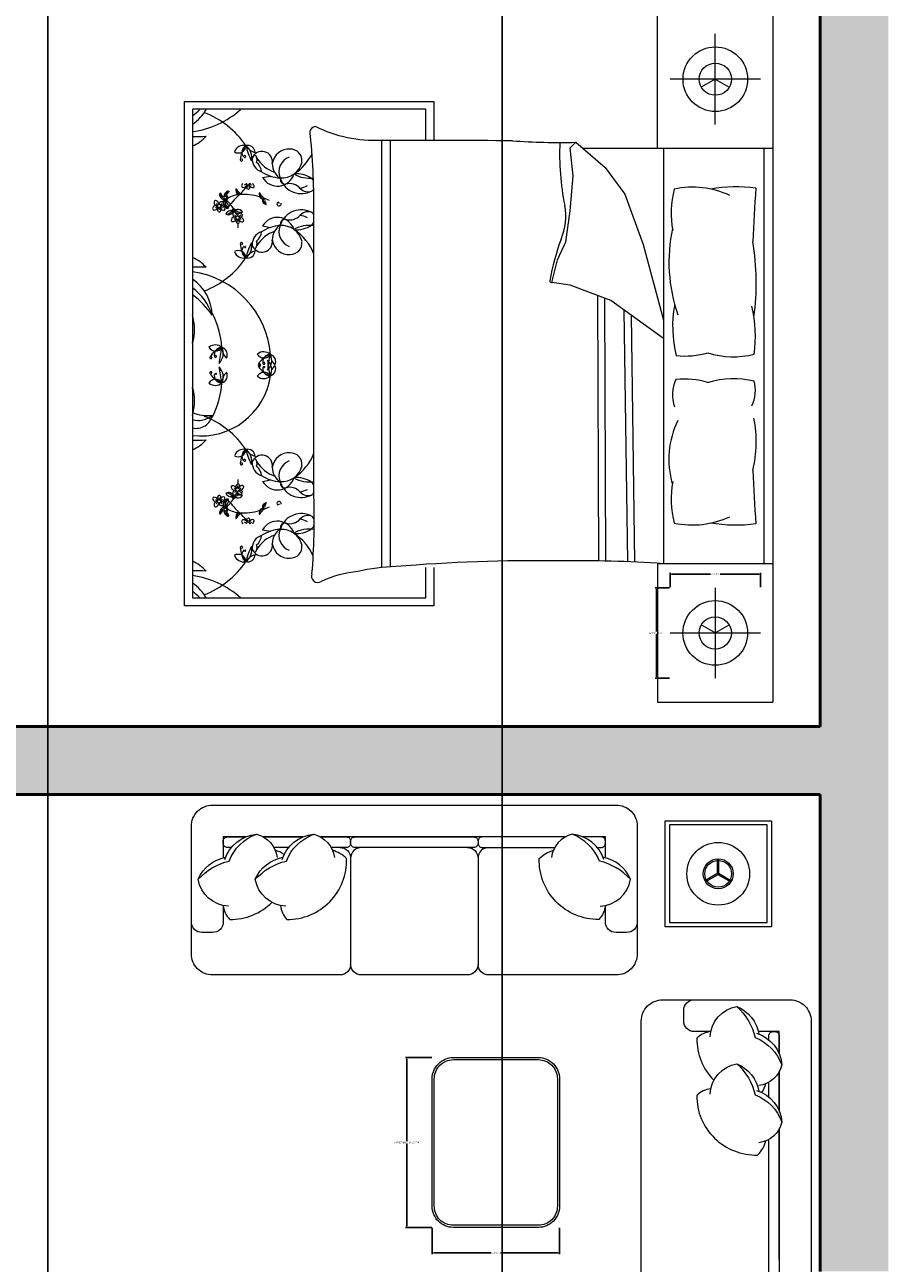
# Model space of a CAD drawing. Units: inches. Extents: x -12 to 604, y -566 to 58.
# Tile 6 of 12: x 166 to 280, y -189 to -25. Entities that reach past the tile are written whole.
import ezdxf

# ---------------------------------------------------------------- set-up
doc = ezdxf.new("R2010")
doc.units = ezdxf.units.IN
doc.header["$MEASUREMENT"] = 0
for name, color, linetype, lineweight in [('A-ANNO-DIMS', 2, 'Continuous', 18), ('A-FURN', 8, 'Continuous', 18), ('A-WALL', 7, 'Continuous', 50), ('A-WALL-PATT', 18, 'Continuous', 13)]:
    doc.layers.add(name, color=color, linetype=linetype, lineweight=lineweight)
doc.styles.get("Standard").update_dxf_attribs({"font": 'arial.ttf'})
doc.dimstyles.get("Standard").update_dxf_attribs({"dimtxt": 0.18, "dimasz": 0.18, "dimexe": 0.18, "dimexo": 0.0625, "dimgap": 0.09, "dimtad": 0, "dimtih": 1, "dimtoh": 1, "dimdec": 0, "dimzin": 0, "dimdsep": 46, "dimlunit": 3, "dimtxsty": 'Standard', "dimcen": 0.09, "dimadec": 0, "dimazin": 0, "dimtfac": 1, "dimtdec": 0, "dimtofl": 0, "dimtmove": 0, "dimatfit": 3, "dimfxl": 1, "dimtolj": 1, "dimtzin": 0, "dimarcsym": 0})

# ---------------------------------------------------------------- blocks, each defined once
blk = doc.blocks.new('DAY BED1')
at = {"color": 0}
blk.add_line((0.3, 0.25), (0.225, 0.2549), dxfattribs=at)
blk.add_lwpolyline([(-0.3, 0, -0.414214), (-0.4, 0.1), (-0.4, 0.1, 0.317837), (-0.4, 0.1, -0.414214), (-0.4, 0.1), (-0.4, 0.1, 1.186185), (-0.4, 0.1, -0.414214), (-0.4, 0.1), (-0.4, 1.5, -0.414214), (-0.3, 1.6), (0.3, 1.6, -0.414214), (0.4, 1.5), (0.4, 0.1, -0.414214), (0.3, 0)], format="xyb", close=True, dxfattribs=at)
for points in [[(-0.0725, 1.45), (-0.15, 1.45, -0.414214), (-0.2, 1.5), (-0.2, 1.55, -0.414214), (-0.15, 1.6)], [(-0.0756, 1.4249, -0.356772), (0.0505, 1.5682, -0.249542), (0.1543, 1.4384, 9.61688)], [(0.0505, 1.5682, -0.14773), (0.1364, 1.422, -0.213343), (0.2624, 1.2931, -0.178662)], [(-0.0725, 1.4501, 0.165541), (-0.1386, 1.4192, 0.200231), (-0.0581, 1.2207, 0.121523)], [(0.1433, 1.4422, -0.306663), (0.2624, 1.2931, -0.30633), (0.1536, 1.1957, 0.872847)], [(0.25, 1.3448), (0.25, 1.45), (0.1517, 1.45, -0.414214)], [(0.2, 1.4118), (0.2, 1.43, -0.414214), (0.22, 1.45), (0.23, 1.45, -0.414214), (0.25, 1.43)], [(0.25, 1.43), (0.25, 1.3448, -0.414214)], [(-0.0756, 1.1556, -0.356772), (0.0505, 1.2988, -0.249542), (0.1543, 1.169, 9.61688)], [(0.0505, 1.2988, -0.14773), (0.1364, 1.1527, -0.213343), (0.2624, 1.0238, -0.178662)], [(0.25, 1.2616), (0.25, 1.0755, -0.414214)], [(-0.0725, 1.1808, 0.165541), (-0.1386, 1.1498, 0.425989), (0.1479, 0.869, 0.121523), (0.1873, 0.9357, -7.115464)], [(0.1433, 1.1729, -0.306663), (0.2624, 1.0238, -0.30633), (0.1536, 0.9263, 0.872847)], [(0.1678, 1.1631, 0.071865), (0.1873, 1.205, -7.115464)], [(0.2, 1.1425), (0.2, 1.2113, -0.414214)], [(0.25, 0.9923), (0.25, 0.2749, -0.414214), (0.23, 0.2549), (0.22, 0.2549, -0.414214), (0.2, 0.2749), (0.2, 0.9419, -0.414214)], [(0.25, 0.3775), (0.25, 0.3, 0.414214), (0.3, 0.25), (0.35, 0.25, 0.414214), (0.4, 0.3)]]:
    blk.add_lwpolyline(points, format="xyb", dxfattribs=at)
for points in [[(0.25, 1.0755), (0.25, 1.2616)], [(0.25, 0.3775), (0.25, 0.9923)]]:
    blk.add_lwpolyline(points, dxfattribs=at)
blk = doc.blocks.new('SIDE-TABLE-WITH-LAMP')
for p, q in [((6.94, 7.06), (7.93, 8.77)), ((7.09, 6.97), (8.08, 8.68)), ((7.01, 7.1), (5.03, 7.1)), ((7.01, 6.92), (5.03, 6.92)), ((6.94, 6.97), (7.93, 5.26)), ((7.09, 7.06), (8.08, 5.34))]:
    blk.add_line(p, q)
at = {"ltscale": 0.03}
blk.add_lwpolyline([(14.03, 14.03), (14.03, 0), (0, 0), (0, 14.03)], close=True, dxfattribs=at)
blk.add_lwpolyline([(13.46, 0.56), (13.46, 13.46), (0.56, 13.46), (0.56, 0.56)], close=True)
for radius in [4.14, 1.98, 1.77]:
    blk.add_circle((7.01, 7.01), radius)
blk = doc.blocks.new('BEDSIDE-LAMP-217')
for p, q in [((5.97, 11.95), (5.97, 0)), ((0, 5.97), (11.95, 5.97))]:
    blk.add_line(p, q)
for points in [[(5.97, 5.97), (4.13, 7.04)], [(5.97, 5.97), (7.82, 7.04)]]:
    blk.add_lwpolyline(points)
for radius in [4.27, 2.13]:
    blk.add_circle((5.97, 5.97), radius)
blk = doc.blocks.new('COFFEE-TABLE')
at = {"ltscale": 0.03}
for points in [[(0, 2.81), (0, 14.03, -0.414214), (2.81, 16.83), (19.64, 16.83, -0.414214), (22.44, 14.03), (22.44, 2.81, -0.414214), (19.64, 0), (2.81, 0, -0.414214)], [(0.28, 2.81), (0.28, 14.03, -0.414214), (2.81, 16.55), (19.64, 16.55, -0.414214), (22.16, 14.03), (22.16, 2.81, -0.414214), (19.64, 0.28), (2.81, 0.28, -0.414214)]]:
    blk.add_lwpolyline(points, format="xyb", close=True, dxfattribs=at)
blk = doc.blocks.new('*D39')
at = {"layer": 'A-ANNO-DIMS', "color": 0, "lineweight": -2, "transparency": 16777216}
for p, q in [((251.44, -99.54), (249.53, -99.54)), ((249.71, -99.72), (249.71, -105.33)), ((249.71, -111.31), (249.71, -105.69)), ((251.44, -111.49), (249.53, -111.49))]:
    blk.add_line(p, q, dxfattribs=at)
at = {"layer": 'A-ANNO-DIMS', "color": 0, "transparency": 16777216}
for points in [[(249.68, -99.72), (249.74, -99.72), (249.71, -99.54)], [(249.68, -111.31), (249.74, -111.31), (249.71, -111.49)]]:
    blk.add_solid(points, dxfattribs=at)
at = {"layer": 'Defpoints', "color": 0, "transparency": 16777216}
for p in [(249.71, -99.54), (251.5, -99.54), (251.5, -111.49)]:
    blk.add_point(p, dxfattribs=at)
at = {"layer": 'A-ANNO-DIMS', "color": 0, "transparency": 16777216, "insert": (249.71, -105.51), "char_height": 0.18, "attachment_point": 5}
blk.add_mtext('\\A1;LAMP B 1\'-0" TYP.', dxfattribs=at)
blk = doc.blocks.new('*D40')
at = {"layer": 'A-ANNO-DIMS', "color": 0, "lineweight": -2, "transparency": 16777216}
for p, q in [((251.5, -99.48), (251.5, -97.57)), ((251.68, -97.75), (256.85, -97.75)), ((263.27, -97.75), (258.11, -97.75)), ((263.45, -99.48), (263.45, -97.57))]:
    blk.add_line(p, q, dxfattribs=at)
at = {"layer": 'A-ANNO-DIMS', "color": 0, "transparency": 16777216}
for points in [[(251.68, -97.72), (251.68, -97.78), (251.5, -97.75)], [(263.27, -97.72), (263.27, -97.78), (263.45, -97.75)]]:
    blk.add_solid(points, dxfattribs=at)
at = {"layer": 'Defpoints', "color": 0, "transparency": 16777216}
for p in [(263.45, -97.75), (251.5, -99.54), (263.45, -99.54)]:
    blk.add_point(p, dxfattribs=at)
at = {"layer": 'A-ANNO-DIMS', "color": 0, "transparency": 16777216, "insert": (257.48, -97.75), "char_height": 0.18, "attachment_point": 5}
blk.add_mtext('\\A1;1\'-0" TYP.', dxfattribs=at)
blk = doc.blocks.new('*D47')
at = {"layer": 'A-ANNO-DIMS', "color": 0, "lineweight": -2, "transparency": 16777216}
for p, q in [((220.01, -161.6), (216.53, -161.6)), ((216.71, -161.78), (216.71, -172.64)), ((216.71, -183.86), (216.71, -173.01)), ((220.01, -184.04), (216.53, -184.04))]:
    blk.add_line(p, q, dxfattribs=at)
at = {"layer": 'A-ANNO-DIMS', "color": 0, "transparency": 16777216}
for points in [[(216.68, -161.78), (216.74, -161.78), (216.71, -161.6)], [(216.68, -183.86), (216.74, -183.86), (216.71, -184.04)]]:
    blk.add_solid(points, dxfattribs=at)
at = {"layer": 'Defpoints', "color": 0, "transparency": 16777216}
for p in [(220.07, -161.6), (216.71, -184.04), (220.07, -184.04)]:
    blk.add_point(p, dxfattribs=at)
at = {"layer": 'A-ANNO-DIMS', "color": 0, "transparency": 16777216, "insert": (216.71, -172.82), "char_height": 0.18, "attachment_point": 5}
blk.add_mtext('\\A1;COFFEE TABLE 1\'-10 1/2" TYP.', dxfattribs=at)
blk = doc.blocks.new('*D48')
at = {"layer": 'A-ANNO-DIMS', "color": 0, "lineweight": -2, "transparency": 16777216}
for p, q in [((220.07, -184.11), (220.07, -187.59)), ((236.91, -184.11), (236.91, -187.59)), ((220.25, -187.41), (227.86, -187.41)), ((236.73, -187.41), (229.12, -187.41))]:
    blk.add_line(p, q, dxfattribs=at)
at = {"layer": 'A-ANNO-DIMS', "color": 0, "transparency": 16777216}
for points in [[(220.25, -187.38), (220.25, -187.44), (220.07, -187.41)], [(236.73, -187.38), (236.73, -187.44), (236.91, -187.41)]]:
    blk.add_solid(points, dxfattribs=at)
at = {"layer": 'Defpoints', "color": 0, "transparency": 16777216}
for p in [(220.07, -184.04), (236.91, -184.04), (236.91, -187.41)]:
    blk.add_point(p, dxfattribs=at)
at = {"layer": 'A-ANNO-DIMS', "color": 0, "transparency": 16777216, "insert": (228.49, -187.41), "char_height": 0.18, "attachment_point": 5}
blk.add_mtext('\\A1;1\'-5" TYP.', dxfattribs=at)
blk = doc.blocks.new('*D57')
at = {"layer": 'A-ANNO-DIMS', "color": 0, "lineweight": -2, "transparency": 16777216}
for p, q in [((169.32, 12.58), (169.32, -565.59)), ((229.32, 12.58), (229.32, -565.59)), ((169.5, -565.41), (198.99, -565.41)), ((229.14, -565.41), (199.65, -565.41))]:
    blk.add_line(p, q, dxfattribs=at)
at = {"layer": 'A-ANNO-DIMS', "color": 0, "transparency": 16777216}
for points in [[(169.5, -565.38), (169.5, -565.44), (169.32, -565.41)], [(229.14, -565.38), (229.14, -565.44), (229.32, -565.41)]]:
    blk.add_solid(points, dxfattribs=at)
at = {"layer": 'Defpoints', "color": 0, "transparency": 16777216}
for p in [(169.32, 12.64), (229.32, 12.64), (229.32, -565.41)]:
    blk.add_point(p, dxfattribs=at)
at = {"layer": 'A-ANNO-DIMS', "color": 0, "transparency": 16777216, "insert": (199.32, -565.41), "char_height": 0.18, "attachment_point": 5}
blk.add_mtext('\\A1;5\'-0"', dxfattribs=at)

msp = doc.modelspace()

# ---------------------------------------------------------------- hatches: boundary and pattern name
at = {"layer": 'A-WALL-PATT'}
h = msp.add_hatch(color=256, dxfattribs=at)
h.dxf.hatch_style = 1
h.paths.add_polyline_path([(169.32, 11.14), (169.32, 17.14), (160.32, 17.14), (160.32, 11.14), (118.32, 11.14), (118.32, 6.64), (118.32, 2.14), (127.32, 2.14), (169.32, 2.14)])
h.paths.add_polyline_path([(127.32, -13.61), (118.32, -13.61), (118.32, -29.36), (34.82, -29.36), (24.32, -29.36), (24.32, -38.36), (39.32, -38.36), (118.32, -38.36), (118.32, -126.86), (127.32, -126.86), (127.32, -117.86)])
h.paths.add_polyline_path([(82.32, -92.36), (39.32, -92.36), (39.32, -56.22), (30.32, -56.22), (24.32, -56.22), (24.32, -65.22), (30.32, -65.22), (30.32, -113.36), (24.32, -113.36), (24.32, -122.36), (39.32, -122.36), (39.32, -101.36), (82.32, -101.36), (82.32, -96.86)], flags=17)
h.paths.add_polyline_path([(280.32, 11.14), (238.32, 11.14), (238.32, 17.14), (229.32, 17.14), (229.32, 12.64), (229.32, 11.14), (229.32, 2.14), (271.32, 2.14), (271.32, -117.86), (163.32, -117.86), (163.32, -126.86), (271.32, -126.86), (271.32, -189.86), (280.32, -189.86), (280.32, -180.86)])
h.paths.add_polyline_path([(415.32, 17.14), (406.32, 17.14), (406.32, 11.14), (358.32, 11.14), (358.32, -21.86), (367.32, -21.86), (367.32, 2.14), (415.32, 2.14)], flags=17)
h.paths.add_polyline_path([(484.55, -45.86), (448.32, -45.86), (448.32, 2.14), (448.32, 17.14), (439.32, 17.14), (439.32, 12.64), (439.32, 2.14), (439.32, -45.86), (367.32, -45.86), (358.32, -45.86), (358.32, -54.86), (430.32, -54.86), (430.32, -69.59), (430.32, -180.86), (318.82, -180.86), (318.82, -189.86), (318.82, -331.86), (327.82, -331.86), (327.82, -189.86), (439.32, -189.86), (439.32, -180.86), (439.32, -54.86), (483.5, -54.86), (484.55, -54.86)])
h.paths.add_polyline_path([(529.32, 11.14), (481.32, 11.14), (481.32, 17.14), (472.32, 17.14), (472.32, 12.64), (472.32, 2.14), (520.32, 2.14), (520.32, -21.86), (529.32, -21.86)])
h.paths.add_polyline_path([(598.32, -45.86), (582.42, -45.86), (582.42, -50.36), (582.42, -54.86), (589.32, -54.86), (589.32, -99.86), (598.32, -99.86), (604.32, -99.86), (604.32, -90.86), (598.32, -90.86)])
h.paths.add_polyline_path([(598.32, -168.86), (604.32, -168.86), (604.32, -159.86), (589.32, -159.86), (589.32, -180.86), (477.32, -180.86), (477.32, -189.86), (477.32, -259.86), (486.32, -259.86), (486.32, -189.86), (589.32, -189.86), (589.32, -204.86), (598.32, -204.86), (604.32, -204.86), (604.32, -195.86), (598.32, -195.86)])
h.paths.add_polyline_path([(598.32, -244.86), (604.32, -244.86), (604.32, -235.86), (598.32, -235.86), (589.32, -235.86), (589.32, -250.86), (522.32, -250.86), (522.32, -259.86), (589.32, -259.86), (589.32, -274.86), (598.32, -274.86), (604.32, -274.86), (604.32, -265.86), (598.32, -265.86)])
h.paths.add_polyline_path([(598.32, -333.28), (604.32, -333.28), (604.32, -324.28), (598.32, -324.28), (598.32, -321.87), (598.32, -318.28), (604.32, -318.28), (604.32, -309.28), (598.32, -309.28), (589.32, -309.28), (589.32, -341.95), (589.38, -341.95), (589.38, -363.16), (589.32, -381.86), (565.32, -381.86), (565.32, -390.86), (589.32, -390.86), (589.32, -450.86), (598.32, -450.86), (604.32, -450.86), (604.32, -441.86), (598.32, -441.86), (598.32, -390.86), (604.32, -390.86), (604.32, -381.86), (598.32, -381.86)])
h.paths.add_polyline_path([(541.32, -345.86), (424.32, -345.86), (424.32, -354.86), (532.32, -354.86), (532.32, -474.86), (463.39, -474.86), (463.39, -483.86), (553.32, -483.86), (553.32, -474.86), (541.32, -474.86), (541.32, -390.86), (541.32, -381.86)])
h.paths.add_polyline_path([(604.32, -474.86), (589.32, -474.86), (553.32, -474.86), (553.32, -483.86), (598.32, -483.86), (604.32, -483.86)])
h.paths.add_polyline_path([(388.32, -483.86), (388.32, -474.86), (388.32, -460.13), (388.32, -333.86), (388.32, -322.86), (379.32, -322.86), (379.32, -331.86), (379.32, -333.86), (379.32, -474.86), (379.32, -520.86), (344.32, -520.86), (344.32, -529.86), (379.32, -529.86), (388.32, -529.86)])
h.paths.add_polyline_path([(284.32, -520.86), (249.32, -520.86), (249.32, -474.86), (249.32, -368.36), (240.32, -368.36), (240.32, -474.86), (238.52, -474.86), (238.52, -483.86), (240.32, -483.86), (240.32, -529.86), (249.32, -529.86), (284.32, -529.86)])
h.paths.add_polyline_path([(178.82, -474.86), (158.91, -474.86), (158.91, -483.86), (162.32, -483.86), (178.82, -483.86)])
h.paths.add_polyline_path([(84.32, -474.86), (84.32, -366.86), (75.32, -366.86), (75.32, -474.86), (39.32, -474.86), (39.32, -453.86), (24.32, -453.86), (24.32, -462.86), (30.32, -462.86), (30.32, -483.86), (84.32, -483.86)])
h.paths.add_polyline_path([(39.32, -342.86), (75.32, -342.86), (84.32, -342.86), (179.67, -342.86), (179.67, -333.86), (39.32, -333.86), (39.32, -318.86), (24.32, -318.86), (24.32, -327.86), (30.32, -327.86), (30.32, -432.86), (24.32, -432.86), (24.32, -441.86), (30.32, -441.86), (39.32, -441.86)])
h.paths.add_polyline_path([(249.32, -252.86), (115.32, -252.86), (115.32, -225.86), (106.32, -225.86), (106.32, -252.86), (39.32, -252.86), (39.32, -237.86), (24.32, -237.86), (24.32, -246.86), (30.32, -246.86), (30.32, -267.86), (24.32, -267.86), (24.32, -276.86), (39.32, -276.86), (39.32, -261.86), (240.32, -261.86), (240.32, -331.86), (249.32, -331.86), (266.82, -331.86), (266.82, -322.86), (249.32, -322.86)])
h.paths.add_polyline_path([(127.32, -180.86), (39.32, -180.86), (24.32, -180.86), (24.32, -189.86), (39.32, -189.86), (127.32, -189.86)])
h.paths.add_polyline_path([(39.32, -159.86), (24.32, -159.86), (24.32, -168.86), (30.32, -168.86), (30.32, -180.86), (39.32, -180.86)])
h.paths.add_polyline_path([(470.51, -17.27), (512.48, -17.27), (512.48, 5.12), (470.51, 5.12)], flags=9)
h.paths.add_polyline_path([(484.21, -244.26), (526.45, -244.26), (526.45, -221.87), (484.21, -221.87)], flags=24)
h.paths.add_polyline_path([(36.91, -442.88), (83.54, -442.88), (83.54, -420.5), (36.91, -420.5)], flags=25)

# ---------------------------------------------------------------- linework, layer by layer
at = {"layer": 'A-FURN'}
for p, q in [((265.09, -23.23), (265.09, -114.65)), ((187.34, -35.3), (220.28, -35.3)), ((187.34, -101.95), (187.34, -35.3)), ((220.28, -35.3), (220.28, -40.47)), ((188.4, -36.35), (188.4, -100.89)), ((219.22, -36.35), (188.4, -36.35)), ((219.22, -40.46), (219.22, -36.35)), ((213.43, -96.87), (213.43, -40.46)), ((214.57, -96.78), (214.57, -40.46)), ((238.31, -41.44), (239.05, -40.69)), ((239.05, -40.69), (242.93, -44.03)), ((238.68, -45.14), (238.31, -41.44)), ((265.09, -41.51), (240, -41.51)), ((250.65, -41.51), (250.65, -96.37)), ((263.92, -96.37), (263.92, -41.51)), ((242.93, -44.03), (245.52, -47.55)), ((197.67, -45.36), (198.7, -45.16)), ((238.31, -49.77), (238.68, -45.14)), ((245.52, -47.55), (247.93, -54.21)), ((204.45, -87.5), (204.45, -50.38)), ((237.75, -53.84), (238.31, -49.77)), ((197.67, -51.75), (198.7, -51.96)), ((236.64, -56.25), (237.75, -53.84)), ((247.93, -54.21), (250.65, -64.18)), ((235.9, -59.21), (236.64, -56.25)), ((238.31, -59.58), (235.9, -59.21)), ((243.67, -61.62), (238.31, -59.58)), ((242.09, -96.05), (241.95, -60.97)), ((243.03, -96.04), (242.89, -61.32)), ((250.65, -66.63), (243.67, -61.62)), ((245.91, -96.09), (245.44, -62.89)), ((246.85, -96.12), (246.39, -63.57)), ((197.67, -85.49), (198.7, -85.29)), ((197.67, -91.88), (198.7, -92.08)), ((219.22, -100.89), (219.22, -96.86)), ((220.28, -96.88), (220.28, -101.95)), ((188.4, -100.89), (219.22, -100.89)), ((220.28, -101.95), (187.34, -101.95))]:
    msp.add_line(p, q, dxfattribs=at)
for points in [[(249.86, -41.51), (249.86, -23.23), (265.09, -23.23)], [(265.09, -96.37), (249.86, -96.37), (249.86, -114.65), (265.09, -114.65)], [(202.97, -132.46), (197.75, -132.46)], [(237.67, -132.46), (205.31, -132.46)], [(242.96, -135.21), (242.96, -132.46), (240.01, -132.46)]]:
    msp.add_lwpolyline(points, dxfattribs=at)
for points in [[(230.67, -40.5, 0.001242), (213.33, -40.46, -0.127202), (204.68, -38.63)], [(262.82, -46.76, 0.074897), (256.84, -46.88, -0.472817)], [(256.51, -68.51, 0.14099), (262.6, -68.7, 0.235245)], [(256.51, -72.42, -0.14099), (262.6, -72.23, -0.235245)], [(262.82, -91.12, -0.074897), (256.84, -91.01, 0.472817)], [(215.29, -96.76, 0.056112), (210.26, -97.42, 0.095341), (205.42, -98.71)], [(189.15, -138.05, -0.14773), (193.25, -135.64, -0.213343), (196.87, -132.11, -0.178662)], [(195.42, -132.46), (192.47, -132.46), (192.47, -135.21, -0.414214)], [(193.54, -133.86), (193.03, -133.86, -0.414214), (192.47, -133.3), (192.47, -133.02, -0.414214), (193.03, -132.46)], [(192.68, -135.45, -0.306663), (196.87, -132.11, -0.30633), (199.6, -135.16, 0.872847)], [(193.03, -132.46), (195.42, -132.46, -0.414214)], [(196.71, -138.05, -0.14773), (200.81, -135.64, -0.213343), (204.42, -132.11, -0.178662)], [(197.75, -132.46), (202.97, -132.46, -0.414214)], [(200.24, -135.45, -0.306663), (204.42, -132.11, -0.30633), (207.16, -135.16, 0.872847)], [(205.31, -132.46), (208.74, -132.46, -0.414214), (209.3, -133.02), (209.3, -133.3, -0.414214), (208.74, -133.86), (206.72, -133.86, -0.414214)], [(237.67, -132.46), (226.69, -132.46, 0.414214), (226.13, -133.02), (226.13, -133.3, 0.414214), (226.69, -133.86), (236.26, -133.86, 0.414214)], [(242.74, -135.45, 0.306663), (238.56, -132.11, 0.30633), (235.82, -135.16, -0.872847)], [(246.27, -138.05, 0.14773), (242.17, -135.64, 0.213343), (238.56, -132.11, 0.178662)], [(242.4, -132.46), (240.01, -132.46, 0.414214)], [(241.89, -133.86), (242.4, -133.86, 0.414214), (242.96, -133.3), (242.96, -133.02, 0.414214), (242.4, -132.46)], [(201.09, -133.86), (199.16, -133.86, -0.414214)], [(207.89, -133.86, -0.414214), (209.3, -135.26), (209.3, -149.29, -0.414214)], [(210.7, -133.86, 0.414214), (209.3, -135.26)], [(224.72, -133.86, -0.414214), (226.13, -135.26)], [(227.53, -133.86, 0.414214), (226.13, -135.26), (226.13, -149.29, 0.414214)], [(193.17, -141.59, -0.356772), (189.15, -138.05, -0.249542), (192.79, -135.14, 9.61688)], [(200.73, -141.59, -0.356772), (196.71, -138.05, -0.249542), (200.35, -135.14, 9.61688)], [(200.51, -134.76, 0.071865), (199.34, -134.22, -7.115464)], [(200.02, -141.5, 0.165541), (200.89, -143.36, 0.425989), (208.76, -135.32, 0.121523), (206.89, -134.22, -7.115464)], [(242.96, -141.5, -0.165541), (242.09, -143.36, -0.425989), (234.22, -135.32, -0.121523), (236.09, -134.22, 7.115464)], [(242.25, -141.59, 0.356772), (246.27, -138.05, 0.249542), (242.63, -135.14, -9.61688)], [(192.47, -141.51), (192.47, -143.68, -0.414214), (191.06, -145.08), (189.66, -145.08, -0.414214), (188.26, -143.68)], [(192.46, -141.5, 0.165541), (193.33, -143.36, 0.200231), (198.9, -141.1, 0.121523)], [(247.17, -143.68, -0.414214), (245.76, -145.08), (244.36, -145.08, -0.414214), (242.96, -143.68), (242.96, -141.51)]]:
    msp.add_lwpolyline(points, format="xyb", dxfattribs=at)
at = {"layer": 'A-FURN', "ltscale": 0.03}
msp.add_lwpolyline([(247.17, -147.89, -0.414214), (244.36, -150.69), (227.53, -150.69, -0.414214), (226.13, -149.29, -0.414214), (224.72, -150.69), (210.7, -150.69, -0.414214), (209.3, -149.29, -0.414214), (207.89, -150.69), (191.06, -150.69, -0.414214), (188.26, -147.89), (188.26, -131.06, -0.414214), (191.06, -128.25), (244.36, -128.25, -0.414214), (247.17, -131.06)], format="xyb", close=True, dxfattribs=at)
at = {"layer": 'A-FURN'}
msp.add_lwpolyline([(209.86, -132.46), (225.57, -132.46, -0.414214), (226.13, -133.02), (226.13, -133.3, -0.414214), (225.57, -133.86), (209.86, -133.86, -0.414214), (209.3, -133.3), (209.3, -133.02, -0.414214)], format="xyb", close=True, dxfattribs=at)
for centre in [(191.9, -49.12), (194.36, -50.65), (194.36, -86.6), (191.9, -88.12)]:
    msp.add_circle(centre, 0.233, dxfattribs=at)
for centre, radius, start, end in [((184.11, -31.36), 7.25, 306.3036, 316.4814), ((185.19, -33.46), 5.82, 303.4617, 330.1116), ((186.79, -27.47), 11.94, 277.745, 311.8856), ((185.61, -47.89), 11.94, 34.3865, 68.5908), ((204.74, -39.47), 0.844, 93.98, 207.3412), ((186.54, -36.71), 4.85, 292.5547, 318.9546), ((189.15, -23.42), 16.52, 267.4081, 273.6519), ((109.28, -49.29), 95.18, 359.3433, 5.6887), ((236.77, 43.13), 83.86, 265.8294, 271.553), ((271.42, -42.26), 34.51, 177.4519, 191.3392), ((195.18, -42.44), 1.32, 77.7115, 159.0387), ((194.47, -41.12), 0.997, 238.4633, 358.2869), ((197.74, -43.14), 3.02, 138.8402, 177.9352), ((195.92, -42.01), 0.977, 117.6827, 223.7762), ((195.31, -42.6), 0.129, 223.7762, 159.7183), ((195.7, -42.11), 0.99, 2.9516, 103.728), ((203.62, -39.34), 8.35, 192.5173, 207.1824), ((194.36, -42.68), 1.89, 345.4653, 54.2343), ((197.21, -40.09), 2.04, 211.3827, 255.2969), ((197.6, -43.27), 1.37, 350.264, 160.8688), ((196.11, -42.99), 0.841, 333.9755, 53.2681), ((201.12, -43.78), 2.18, 84.9449, 172.8857), ((201.34, -43.14), 1.54, 354.4856, 91.0538), ((198.02, -39.11), 6.92, 303.6671, 333.2997), ((194.87, -43.03), 0.148, 177.9352, 11.4834), ((194.94, -43.02), 0.072, 11.4834, 127.9409), ((198.01, -42.94), 1.71, 175.969, 254.3045), ((195.73, -44.79), 1.82, 6.1662, 51.5825), ((200.62, -40.55), 4.32, 211.2614, 251.7045), ((201.6, -43.4), 2.66, 182.3591, 234.0401), ((201.95, -44.63), 2.12, 111.5819, 201.4221), ((200.2, -42.67), 2.75, 265.2933, 346.921), ((200.27, -40.51), 4.91, 236.2883, 266.5076), ((199.64, -44.23), 2.27, 209.9085, 343.1337), ((200.6, -45.67), 0.567, 167.3041, 285.1471), ((202.13, -48.39), 3.53, 122.7011, 126.3445), ((202.79, -44.58), 2.91, 199.2822, 299.1751), ((203.78, -41.65), 3.79, 238.8218, 279.1554), ((202.13, -48.39), 3.53, 55.785, 94.7304), ((203.44, -46.34), 1.1, 30.0293, 52.325), ((192.24, -47.62), 0.26, 124.3538, 214.3923), ((192.8, -47.44), 0.704, 176.9701, 248.2913), ((197.82, -43.73), 6.8, 212.6784, 216.3746), ((193.2, -47.8), 0.606, 122.8155, 187.3992), ((193.47, -47.87), 0.704, 109.4799, 177.6828), ((193.09, -47.43), 0.26, 56.8636, 146.9021), ((198.82, -51.09), 6.8, 145.1882, 148.8844), ((196.72, -46.91), 2.58, 178.3264, 187.1302), ((193.94, -47.27), 0.48, 11.3256, 64.4621), ((195.56, -46.58), 1.45, 190.2588, 210.656), ((194.6, -47.17), 0.439, 188.3432, 274.2869), ((194.98, -46.92), 0.766, 210.656, 242.6341), ((195.56, -46.26), 1.47, 218.2101, 226.3071), ((194.47, -47.5), 0.186, 325.7657, 67.4417), ((188.69, -41.27), 8.68, 313.1541, 322.0459), ((195.07, -46.49), 0.179, 142.4737, 265.053), ((195.31, -46.45), 0.384, 127.7621, 169.0403), ((195.11, -46.12), 0.541, 265.053, 338.3618), ((195.82, -46.86), 0.707, 113.4276, 137.6104), ((195.74, -46.13), 0.233, 183.2768, 356.7232), ((195.91, -46.55), 0.381, 139.7889, 227.6792), ((195.79, -46.69), 0.201, 227.6792, 350.3487), ((195.01, -46.55), 0.762, 353.0852, 15.7171), ((195.51, -46.64), 0.481, 350.3487, 43.6538), ((196.41, -46.14), 0.56, 198.7263, 262.5032), ((195.96, -46.4), 0.222, 1.1081, 91.8675), ((196.38, -46.52), 0.18, 255.2356, 54.9248), ((196.1, -46.45), 0.388, 11.5637, 52.6358), ((199.8, -47.45), 2.58, 178.3264, 187.1302), ((197.01, -47.81), 0.48, 11.3256, 64.4621), ((198.64, -47.12), 1.45, 190.2588, 210.656), ((201.23, -48.03), 1.87, 41.5653, 105.1471), ((202.27, -44.14), 2.63, 277.436, 299.9149), ((203.66, -45.88), 1.37, 221.5653, 293.8354), ((203.44, -46.34), 1.1, 314.4517, 333.558), ((263.89, -50.03), 12.25, 165.1039, 191.0369), ((254.45, -58.41), 11.78, 65.1316, 101.7583), ((1132.9, -97.16), 871.54, 176.68521, 177.14978), ((191.47, -49.44), 0.384, 61.2196, 169.0403), ((191.73, -48.65), 0.46, 157.4086, 261.4386), ((191.47, -48.63), 0.231, 58.0499, 135.6268), ((191.71, -48.78), 0.154, 172.906, 277.132), ((191.2, -49.06), 0.734, 14.7558, 58.0499), ((192.23, -48.87), 0.318, 36.1046, 181.4281), ((192.62, -47.66), 0.606, 190.3057, 287.1958), ((192.04, -48.62), 0.32, 270.0645, 331.1507), ((192.32, -48.69), 0.366, 221.8413, 265.7877), ((192.31, -48.83), 0.228, 263.7526, 41.7054), ((192.26, -49.45), 0.388, 11.5637, 86.365), ((192.56, -47.61), 0.269, 216.3746, 291.7548), ((194.94, -51.39), 3.8, 124.0033, 132.4917), ((191.04, -51.87), 4.06, 63.7819, 68.2913), ((193.2, -48.74), 0.645, 128.3208, 208.8162), ((193.32, -48.7), 0.771, 207.7043, 254.3516), ((192.74, -48.05), 0.203, 289.3605, 111.7548), ((192.89, -48.05), 0.203, 221.8703, 44.2646), ((193.81, -48.64), 1.06, 157.2305, 229.0635), ((193.45, -48.29), 0.625, 174.4544, 220.6188), ((189.9, -51.78), 4.55, 30.544, 49.818), ((193.23, -47.72), 0.269, 148.8844, 224.2646), ((192.41, -49.18), 0.751, 340.0041, 40.6188), ((194.94, -51.39), 3.8, 94.756, 119.2041), ((203.03, -56.85), 12.49, 132.2412, 142.1744), ((195.13, -55.16), 7.57, 73.5842, 93.8277), ((197.67, -47.71), 0.439, 188.3432, 274.2869), ((198.06, -47.47), 0.766, 210.656, 242.6341), ((198.64, -46.81), 1.47, 218.2101, 226.3071), ((197.55, -48.04), 0.186, 325.7657, 67.4417), ((198.07, -48.38), 0.439, 147.5332, 233.4768), ((198.47, -48.16), 0.766, 179.1859, 211.164), ((197.72, -48.33), 0.186, 354.3784, 96.0543), ((195.13, -55.16), 7.57, 63.0032, 69.8941), ((199.3, -46.63), 2.58, 234.6898, 243.4936), ((199.05, -47.81), 1.45, 211.164, 231.5612), ((199.33, -47.96), 1.47, 195.5129, 203.6099), ((197.67, -48.92), 0.48, 357.3579, 50.4944), ((199.74, -48.82), 0.176, 12.7051, 190.4384), ((199.84, -48.8), 0.287, 190.4384, 10.4136), ((230.29, -50.51), 7.44, 336.2616, 11.3392), ((191.24, -49.48), 0.179, 142.4737, 265.053), ((191.27, -49.12), 0.541, 265.053, 338.3618), ((191.98, -49.86), 0.707, 113.4276, 137.6104), ((192.07, -49.54), 0.381, 139.7889, 227.6792), ((191.95, -49.68), 0.201, 227.6792, 350.3487), ((191.18, -49.54), 0.762, 353.0852, 15.7171), ((191.68, -49.63), 0.481, 350.3487, 43.6538), ((192.57, -49.13), 0.56, 198.7263, 262.5032), ((192.12, -49.39), 0.222, 1.1081, 91.8675), ((192.54, -49.51), 0.18, 255.2356, 54.9248), ((192.82, -49.14), 1.06, 270.278, 342.111), ((193.53, -50.47), 0.751, 98.7227, 159.3375), ((193.15, -49.5), 0.771, 244.9899, 291.6373), ((193.32, -49.11), 0.625, 278.7227, 324.8872), ((193.21, -49.61), 0.645, 290.5253, 358.5375), ((193.93, -50.96), 0.384, 61.2196, 169.0403), ((194.18, -50.17), 0.46, 157.4086, 261.4386), ((193.92, -50.16), 0.231, 58.0499, 135.6268), ((194.47, -49.43), 0.645, 182.8499, 266.1226), ((194.22, -48.97), 0.625, 231.7607, 277.9252), ((194.7, -48.86), 1.06, 214.5369, 286.3699), ((194.16, -50.3), 0.154, 172.906, 277.132), ((193.65, -50.58), 0.734, 14.7558, 58.0499), ((189.9, -51.78), 4.55, 23.0501, 23.8477), ((194.41, -50.34), 0.751, 37.3105, 97.9252), ((194.68, -50.39), 0.318, 36.1046, 181.4281), ((194.49, -49.31), 0.771, 265.0106, 311.658), ((194.5, -50.14), 0.32, 270.0645, 331.1507), ((194.77, -50.22), 0.366, 221.8413, 265.7877), ((194.58, -50.92), 0.222, 1.1081, 91.8675), ((194.77, -50.35), 0.228, 263.7526, 41.7054), ((194.72, -50.97), 0.388, 11.5637, 86.365), ((199.64, -52.89), 2.27, 16.8663, 150.0915), ((202.79, -52.53), 2.91, 60.8249, 160.7178), ((201.23, -49.09), 1.87, 254.8529, 318.4347), ((202.27, -52.97), 2.63, 60.0851, 82.564), ((203.66, -51.24), 1.37, 66.1646, 138.4347), ((203.44, -50.78), 1.1, 23.229, 45.5483), ((193.69, -51), 0.179, 142.4737, 265.053), ((193.72, -50.64), 0.541, 265.053, 338.3618), ((194.44, -51.38), 0.707, 113.4276, 137.6104), ((194.53, -51.07), 0.381, 139.7889, 227.6792), ((194.41, -51.2), 0.201, 227.6792, 350.3487), ((193.63, -51.06), 0.762, 353.0852, 15.7171), ((189.9, -51.78), 4.55, 357.1071, 4.7585), ((194.13, -51.15), 0.481, 350.3487, 43.6538), ((195.02, -50.66), 0.56, 198.7263, 262.5032), ((195, -51.04), 0.18, 255.2356, 54.9248), ((200.27, -56.61), 4.91, 93.4924, 123.7117), ((201.6, -53.72), 2.66, 125.9599, 177.6409), ((201.95, -52.48), 2.12, 158.5779, 248.4181), ((200.2, -54.45), 2.75, 13.079, 94.7067), ((200.6, -51.45), 0.567, 74.8529, 192.6959), ((202.13, -48.73), 3.53, 233.6555, 237.2989), ((203.78, -55.47), 3.79, 79.7133, 121.1782), ((202.13, -48.73), 3.53, 265.2696, 304.215), ((198.02, -58.01), 6.92, 21.4941, 56.3329), ((203.44, -50.78), 1.1, 307.675, 336.7144), ((272.6, -56.48), 21.25, 168.0397, 199.2615), ((194.87, -54.09), 0.148, 348.5166, 182.0648), ((194.36, -54.44), 1.89, 305.7657, 14.5347), ((203.62, -57.78), 8.35, 152.8176, 167.4827), ((198.01, -54.17), 1.71, 105.6955, 184.031), ((197.6, -53.85), 1.37, 199.1312, 9.736), ((196.11, -54.13), 0.841, 306.7319, 26.0245), ((195.73, -52.33), 1.82, 308.4175, 353.8338), ((200.62, -56.57), 4.32, 108.2955, 148.7386), ((201.12, -53.34), 2.18, 187.1143, 275.0551), ((201.34, -53.98), 1.54, 268.9462, 5.5144), ((270.45, -65.56), 35.46, 160.1194, 169.3383), ((229.73, -59.29), 33.16, 352.2196, 9.497), ((194.47, -56), 0.997, 1.7131, 121.5367), ((195.18, -54.68), 1.32, 200.9613, 282.2885), ((197.74, -53.98), 3.02, 182.0648, 221.1598), ((194.94, -54.1), 0.072, 232.0591, 348.5166), ((195.92, -55.1), 0.977, 136.2238, 242.3173), ((195.36, -54.53), 0.0778, 200.2667, 136.2271), ((195.7, -55.01), 0.99, 256.272, 357.0484), ((197.21, -57.03), 2.04, 104.7031, 148.6173), ((186.54, -60.4), 4.85, 41.0454, 67.4453), ((189.15, -73.7), 16.52, 86.3481, 92.5919), ((185.61, -49.23), 11.94, 291.4092, 325.6135), ((186.79, -69.65), 11.94, 4.4623, 82.255), ((185.19, -63.66), 5.82, 1.272, 56.5383), ((184.11, -65.76), 7.25, 17.8504, 53.6964), ((235.83, -59), 0.221, 178.8623, 289.7536), ((182.07, -69.57), 10.78, 34.0123, 54.053), ((182.12, -65.4), 6.56, 343.5431, 17.0202), ((180.4, -68.74), 11.94, 4.4623, 27.4146), ((267.96, -65.08), 16.12, 169.8617, 193.6238), ((246.49, -66.29), 16.29, 351.5249, 13.96), ((178.74, -68), 9.71, 4.3787, 5.6357), ((172.09, -73.11), 17.35, 19.7217, 19.9028), ((191.41, -68.79), 1.32, 47.7873, 129.1145), ((191.45, -67.29), 0.997, 208.5391, 328.3627), ((193.28, -70.67), 3.02, 108.9159, 148.011), ((192.26, -68.78), 0.977, 87.7585, 193.852), ((200.27, -70.31), 8.35, 162.593, 177.2582), ((190.58, -68.59), 1.89, 315.5411, 24.3101), ((194.34, -67.76), 2.04, 181.4585, 225.3727), ((192.02, -68.76), 0.99, 333.0274, 73.8037), ((197.81, -69.7), 1.32, 47.7873, 129.1145), ((197.85, -68.2), 0.997, 208.5391, 328.3627), ((253.45, -57.74), 11.2, 264.0129, 285.8293), ((190.84, -69.14), 0.148, 148.011, 341.5592), ((190.92, -69.17), 0.072, 341.5592, 98.0167), ((191.44, -68.99), 0.129, 193.852, 129.9245), ((197.24, -70.06), 0.148, 148.011, 341.5592), ((197.24, -70.23), 0.148, 18.4408, 211.989), ((199.67, -71.58), 3.02, 108.9159, 148.011), ((199.67, -68.71), 3.02, 211.989, 251.0841), ((197.31, -70.08), 0.072, 341.5592, 98.0167), ((197.31, -70.21), 0.072, 261.9833, 18.4408), ((198.66, -69.7), 0.977, 87.7585, 193.852), ((197.83, -69.9), 0.129, 193.852, 129.9245), ((197.88, -70.38), 0.0778, 230.1909, 166.0209), ((196.98, -69.5), 1.89, 315.5411, 24.3101), ((206.67, -71.22), 8.35, 162.593, 177.2582), ((196.98, -70.79), 1.89, 335.6899, 44.4589), ((206.67, -69.07), 8.35, 182.7418, 197.407), ((198.42, -69.67), 0.99, 333.0274, 73.8037), ((200.73, -68.67), 2.04, 181.4585, 225.3727), ((198.42, -70.62), 0.99, 286.1963, 26.9726), ((200.73, -71.62), 2.04, 134.6273, 178.5415), ((189.55, -70.25), 9.24, 262.8636, 351.8197), ((190.84, -71.15), 0.148, 18.4408, 211.989), ((193.28, -69.63), 3.02, 211.989, 251.0841), ((190.92, -71.12), 0.072, 261.9833, 18.4408), ((192.26, -71.51), 0.977, 166.148, 272.2415), ((191.49, -71.29), 0.0778, 230.1909, 166.0209), ((200.27, -69.98), 8.35, 182.7418, 197.407), ((190.58, -71.71), 1.89, 335.6899, 44.4589), ((194.34, -72.53), 2.04, 134.6273, 178.5415), ((192.02, -71.53), 0.99, 286.1963, 26.9726), ((197.85, -72.09), 0.997, 31.6373, 151.4609), ((197.81, -70.59), 1.32, 230.8855, 312.2127), ((198.66, -70.59), 0.977, 166.148, 272.2415), ((182.12, -74.89), 6.56, 342.9798, 16.4569), ((178.74, -72.29), 9.71, 354.3643, 355.6213), ((172.09, -67.18), 17.35, 340.0972, 340.2783), ((191.45, -73.01), 0.997, 31.6373, 151.4609), ((191.41, -71.5), 1.32, 230.8855, 312.2127), ((180.4, -71.55), 11.94, 332.5854, 355.5377), ((256.68, -74.1), 4.85, 155.0183, 198.5407), ((253.45, -83.19), 11.2, 74.1707, 95.9871), ((258.26, -73.49), 4.52, 333.3437, 16.1026), ((190.39, -71.45), 5.35, 248.117, 276.6195), ((188.91, -76.35), 2.14, 256.3898, 349.0739), ((189.2, -74.74), 2.71, 252.8609, 311.9049), ((185.61, -88.02), 11.94, 34.3865, 68.5908), ((262.98, -82.57), 11.64, 153.8761, 196.1746), ((246.82, -80.27), 16.07, 346.3427, 11.1841), ((189.15, -63.54), 16.52, 267.4081, 273.6519), ((186.54, -76.84), 4.85, 292.5547, 318.9546), ((195.18, -82.57), 1.32, 77.7115, 159.0387), ((194.47, -81.25), 0.997, 238.4633, 358.2869), ((197.74, -83.26), 3.02, 138.8402, 177.9352), ((195.92, -82.14), 0.977, 117.6827, 223.7762), ((195.7, -82.24), 0.99, 2.9516, 103.728), ((197.21, -80.21), 2.04, 211.3827, 255.2969), ((194.36, -82.81), 1.89, 345.4653, 54.2343), ((203.62, -79.47), 8.35, 192.5173, 207.1824), ((201.12, -83.9), 2.18, 84.9449, 172.8857), ((201.34, -83.27), 1.54, 354.4856, 91.0538), ((198.02, -79.24), 6.92, 303.6671, 338.5059), ((194.87, -83.16), 0.148, 177.9352, 11.4834), ((194.94, -83.14), 0.072, 11.4834, 127.9409), ((195.31, -82.73), 0.129, 223.7762, 159.7183), ((197.6, -83.4), 1.37, 350.264, 160.8688), ((198.01, -83.07), 1.71, 175.969, 254.3045), ((196.11, -83.12), 0.841, 333.9755, 53.2681), ((200.62, -80.68), 4.32, 211.2614, 251.7045), ((201.95, -84.76), 2.12, 111.5819, 201.4221), ((200.2, -82.79), 2.75, 265.2933, 346.921), ((195.73, -84.92), 1.82, 6.1662, 51.5825), ((200.27, -80.64), 4.91, 236.2883, 266.5076), ((199.64, -84.36), 2.27, 209.9085, 343.1337), ((201.6, -83.52), 2.66, 182.3591, 234.0401), ((203.78, -81.78), 3.79, 238.8218, 280.2867), ((202.13, -88.51), 3.53, 55.785, 94.7304), ((1132.9, -40.72), 871.54, 182.85022, 183.31479), ((193.69, -86.25), 0.179, 94.947, 217.5263), ((193.93, -86.28), 0.384, 190.9597, 298.7804), ((193.72, -86.61), 0.541, 21.6382, 94.947), ((194.18, -87.07), 0.46, 98.5614, 202.5914), ((194.44, -85.87), 0.707, 222.3896, 246.5724), ((194.53, -86.18), 0.381, 132.3208, 220.2111), ((194.41, -86.04), 0.201, 9.6513, 132.3208), ((193.63, -86.18), 0.762, 344.2829, 6.9148), ((189.9, -85.47), 4.55, 355.2415, 2.8929), ((194.13, -86.09), 0.481, 316.3462, 9.6513), ((195.02, -86.59), 0.56, 97.4968, 161.2737), ((194.77, -87.03), 0.366, 94.2123, 138.1587), ((194.58, -86.33), 0.222, 268.1325, 358.8919), ((194.72, -86.28), 0.388, 273.635, 348.4363), ((194.77, -86.89), 0.228, 318.2946, 96.2474), ((195, -86.21), 0.18, 305.0752, 104.7644), ((200.6, -85.8), 0.567, 167.3041, 285.1471), ((202.13, -88.51), 3.53, 122.7011, 126.3445), ((202.79, -84.71), 2.91, 199.2822, 299.1751), ((201.23, -88.15), 1.87, 41.5653, 105.1471), ((202.27, -84.27), 2.63, 277.436, 299.9149), ((203.44, -86.47), 1.1, 23.2856, 52.325), ((263.89, -87.86), 12.25, 168.9631, 194.8961), ((191.24, -87.77), 0.179, 94.947, 217.5263), ((191.47, -87.8), 0.384, 190.9597, 298.7804), ((191.27, -88.13), 0.541, 21.6382, 94.947), ((191.73, -88.6), 0.46, 98.5614, 202.5914), ((191.98, -87.39), 0.707, 222.3896, 246.5724), ((191.71, -88.47), 0.154, 82.868, 187.094), ((192.07, -87.7), 0.381, 132.3208, 220.2111), ((191.95, -87.57), 0.201, 9.6513, 132.3208), ((191.18, -87.7), 0.762, 344.2829, 6.9148), ((191.68, -87.61), 0.481, 316.3462, 9.6513), ((192.57, -88.11), 0.56, 97.4968, 161.2737), ((192.32, -88.55), 0.366, 94.2123, 138.1587), ((192.04, -88.63), 0.32, 28.8493, 89.9355), ((192.12, -87.85), 0.222, 268.1325, 358.8919), ((192.26, -87.8), 0.388, 273.635, 348.4363), ((192.31, -88.41), 0.228, 318.2946, 96.2474), ((192.54, -87.73), 0.18, 305.0752, 104.7644), ((193.2, -88.5), 0.645, 151.1838, 231.6792), ((193.32, -88.55), 0.771, 105.6484, 152.2957), ((193.81, -88.61), 1.06, 130.9365, 202.7695), ((193.15, -87.74), 0.771, 68.3627, 115.0101), ((192.82, -88.1), 1.06, 17.889, 89.722), ((193.53, -86.78), 0.751, 200.6625, 261.2773), ((189.9, -85.47), 4.55, 310.182, 329.456), ((192.41, -88.06), 0.751, 319.3812, 19.9959), ((203.03, -80.39), 12.49, 217.8256, 227.7588), ((193.32, -88.14), 0.625, 35.1128, 81.2773), ((193.21, -87.63), 0.645, 1.4625, 69.4747), ((193.92, -87.09), 0.231, 224.3732, 301.9501), ((194.47, -87.81), 0.645, 93.8774, 177.1501), ((194.7, -88.38), 1.06, 73.6301, 145.4631), ((194.22, -88.27), 0.625, 82.0748, 128.2393), ((194.16, -86.94), 0.154, 82.868, 187.094), ((193.65, -86.66), 0.734, 301.9501, 345.2442), ((189.9, -85.47), 4.55, 336.1523, 336.9499), ((194.41, -86.91), 0.751, 262.0748, 322.6895), ((194.68, -86.86), 0.318, 178.5719, 323.8954), ((194.49, -87.94), 0.771, 48.342, 94.9894), ((194.5, -87.11), 0.32, 28.8493, 89.9355), ((199.3, -90.61), 2.58, 116.5064, 125.3102), ((199.05, -89.44), 1.45, 128.4388, 148.836), ((197.67, -88.33), 0.48, 309.5056, 2.6421), ((199.84, -88.44), 0.287, 349.5864, 169.5616), ((203.66, -86), 1.37, 221.5653, 293.8354), ((115.53, -90.3), 88.97, 355.2402, 1.8035), ((203.44, -86.47), 1.1, 314.4517, 336.7144), ((191.47, -88.61), 0.231, 224.3732, 301.9501), ((191.2, -88.18), 0.734, 301.9501, 345.2442), ((192.23, -88.38), 0.318, 178.5719, 323.8954), ((192.24, -89.62), 0.26, 145.6077, 235.6462), ((192.62, -89.58), 0.606, 72.8042, 169.6943), ((192.8, -89.8), 0.704, 111.7087, 183.0299), ((197.82, -93.51), 6.8, 143.6254, 147.3216), ((192.56, -89.64), 0.269, 68.2452, 143.6254), ((194.94, -85.86), 3.8, 227.5083, 235.9967), ((191.04, -85.38), 4.06, 291.7087, 296.2181), ((193.2, -89.45), 0.606, 172.6008, 237.1845), ((192.74, -89.2), 0.203, 248.2452, 70.6395), ((192.89, -89.2), 0.203, 315.7354, 138.1297), ((193.47, -89.37), 0.704, 182.3172, 250.5201), ((193.45, -88.96), 0.625, 139.3812, 185.5456), ((193.09, -89.82), 0.26, 213.0979, 303.1364), ((193.23, -89.53), 0.269, 135.7354, 211.1156), ((198.82, -86.15), 6.8, 211.1156, 214.8118), ((194.94, -85.86), 3.8, 240.7959, 265.244), ((195.56, -90.67), 1.45, 149.344, 169.7412), ((194.6, -90.08), 0.439, 85.7131, 171.6568), ((194.98, -90.32), 0.766, 117.3659, 149.344), ((195.56, -90.98), 1.47, 133.6929, 141.7899), ((194.47, -89.75), 0.186, 292.5583, 34.2343), ((195.13, -82.09), 7.57, 266.1723, 286.4158), ((188.69, -95.97), 8.68, 37.9541, 46.8459), ((198.64, -90.12), 1.45, 149.344, 169.7412), ((199.8, -89.79), 2.58, 172.8698, 181.6736), ((197.01, -89.43), 0.48, 295.5379, 348.6744), ((197.67, -89.53), 0.439, 85.7131, 171.6568), ((198.06, -89.78), 0.766, 117.3659, 149.344), ((198.64, -90.44), 1.47, 133.6929, 141.7899), ((197.55, -89.2), 0.186, 292.5583, 34.2343), ((198.07, -88.86), 0.439, 126.5232, 212.4668), ((198.47, -89.09), 0.766, 148.836, 180.8141), ((197.72, -88.91), 0.186, 263.9457, 5.6216), ((195.13, -82.09), 7.57, 290.1059, 296.9968), ((199.33, -89.29), 1.47, 156.3901, 164.4871), ((199.74, -88.42), 0.176, 169.5616, 347.2949), ((202.79, -92.66), 2.91, 60.8249, 160.7178), ((196.72, -90.34), 2.58, 172.8698, 181.6736), ((193.94, -89.98), 0.48, 295.5379, 348.6744), ((195.07, -90.76), 0.179, 94.947, 217.5263), ((195.31, -90.79), 0.384, 190.9597, 232.2379), ((195.11, -91.12), 0.541, 21.6382, 94.947), ((195.82, -90.38), 0.707, 222.3896, 246.5724), ((195.74, -91.11), 0.233, 3.2768, 176.7232), ((195.91, -90.69), 0.381, 132.3208, 220.2111), ((195.79, -90.56), 0.201, 9.6513, 132.3208), ((195.01, -90.7), 0.762, 344.2829, 6.9148), ((195.51, -90.6), 0.481, 316.3462, 9.6513), ((196.41, -91.1), 0.56, 97.4968, 161.2737), ((195.96, -90.84), 0.222, 268.1325, 358.8919), ((196.38, -90.72), 0.18, 305.0752, 104.7644), ((196.1, -90.79), 0.388, 307.3642, 348.4363), ((199.64, -93.01), 2.27, 16.8663, 150.0915), ((200.6, -91.57), 0.567, 74.8529, 192.6959), ((201.23, -89.22), 1.87, 254.8529, 318.4347), ((202.27, -93.1), 2.63, 60.0851, 82.564), ((203.66, -91.37), 1.37, 66.1646, 138.4347), ((203.44, -90.9), 1.1, 307.675, 342.5814), ((203.44, -90.9), 1.1, 16.6343, 45.5483), ((254.45, -79.47), 11.78, 258.2417, 294.8684), ((198.01, -94.3), 1.71, 105.6955, 184.031), ((195.73, -92.46), 1.82, 308.4175, 353.8338), ((200.62, -96.69), 4.32, 108.2955, 148.7386), ((200.27, -96.73), 4.91, 93.4924, 123.7117), ((201.6, -93.85), 2.66, 125.9599, 177.6409), ((201.95, -92.61), 2.12, 158.5779, 248.4181), ((200.2, -94.58), 2.75, 13.079, 94.7067), ((202.13, -88.86), 3.53, 233.6555, 237.2989), ((203.78, -95.59), 3.79, 79.249, 121.1782), ((202.13, -88.86), 3.53, 265.2696, 304.215), ((198.02, -98.13), 6.92, 23.6453, 56.3329), ((194.87, -94.21), 0.148, 348.5166, 182.0648), ((197.74, -94.11), 3.02, 182.0648, 221.1598), ((194.94, -94.23), 0.072, 232.0591, 348.5166), ((195.92, -95.23), 0.977, 136.2238, 242.3173), ((195.36, -94.66), 0.0778, 200.2667, 136.2271), ((203.62, -97.91), 8.35, 152.8176, 167.4827), ((194.36, -94.56), 1.89, 305.7657, 14.5347), ((197.6, -93.97), 1.37, 199.1312, 9.736), ((196.11, -94.25), 0.841, 306.7319, 26.0245), ((201.12, -93.47), 2.18, 187.1143, 275.0551), ((201.34, -94.1), 1.54, 268.9462, 5.5144), ((186.54, -100.53), 4.85, 41.0454, 67.4453), ((185.61, -89.35), 11.94, 291.4092, 325.6135), ((194.47, -96.13), 0.997, 1.7131, 121.5367), ((195.18, -94.8), 1.32, 200.9613, 282.2885), ((197.21, -97.16), 2.04, 104.7031, 148.6173), ((195.7, -95.13), 0.99, 256.272, 357.0484), ((233.5, -310.28), 214.3, 89.1145, 94.8735), ((239.47, -260.27), 164.28, 86.1, 90.9282), ((189.15, -113.83), 16.52, 86.3481, 92.5919), ((186.79, -109.78), 11.94, 48.1144, 82.255), ((204.96, -98.02), 0.833, 156.5219, 303.8264), ((185.19, -103.79), 5.82, 29.8884, 56.5383), ((184.11, -105.88), 7.25, 43.5186, 53.6964)]:
    msp.add_arc(centre, radius, start, end, dxfattribs=at)
at = {"layer": 'A-WALL'}
for p, q in [((271.32, 2.14), (271.32, -117.86)), ((163.32, -117.86), (271.32, -117.86)), ((163.32, -126.86), (271.32, -126.86)), ((271.32, -126.86), (271.32, -189.86))]:
    msp.add_line(p, q, dxfattribs=at)

# ---------------------------------------------------------------- block references
at = {"layer": 'A-FURN'}
for name, p, rotation in [('BEDSIDE-LAMP-217', (263.45, -26.4), 180), ('SIDE-TABLE-WITH-LAMP', (250.85, -130.32), 269.9999999999988), ('COFFEE-TABLE', (220.07, -161.6), 269.9999999999988)]:
    msp.add_blockref(name, p, dxfattribs=dict(at, rotation=rotation))
msp.add_blockref('BEDSIDE-LAMP-217', (251.5, -111.49), dxfattribs=at)
at = {"layer": 'A-FURN', "ltscale": 0.03, "xscale": 28.05029504973475, "yscale": 28.05029504973475, "zscale": 28.05029504973475}
msp.add_blockref('DAY BED1', (258.92, -198.85), dxfattribs=at)

# ---------------------------------------------------------------- dimensions: what is measured, and where the dimension line sits
at = {"layer": 'A-ANNO-DIMS'}
dim = msp.add_linear_dim(base=(229.32, -565.41), p1=(169.32, 12.64), p2=(229.32, 12.64), dimstyle='Standard', override={"dimdec": 1, "dimlfac": 1, "dimrnd": 0, "dimzin": 1, "dimdsep": 46, "dimlunit": 4, "dimfrac": 2}, dxfattribs=at)
dim.commit()
dim.dimension.update_dxf_attribs({"geometry": '*D57', "text_midpoint": (199.32, -565.41)})
for base, p1, p2, picture, middle in [((263.4491, -97.7468), (251.5026, -99.5388), (263.4491, -99.5388), '*D40', (257.4758, -97.7468)), ((236.91, -187.41), (220.07, -184.04), (236.91, -184.04), '*D48', (228.49, -187.41))]:
    dim = msp.add_linear_dim(base=base, p1=p1, p2=p2, text='<> TYP.', dimstyle='Standard', override={"dimdec": 1, "dimlfac": 1, "dimrnd": 0, "dimzin": 1, "dimdsep": 46, "dimlunit": 4, "dimfrac": 2}, dxfattribs=at)
    dim.commit()
    dim.dimension.update_dxf_attribs({"geometry": picture, "text_midpoint": middle})
for base, p1, p2, angle, text, picture, middle in [((249.7106, -99.5388), (251.5026, -111.4853), (251.5026, -99.5388), 90, 'LAMP B <> TYP.', '*D39', (249.7106, -105.5121)), ((216.71, -184.04), (220.07, -161.6), (220.07, -184.04), 270, 'COFFEE TABLE <> TYP.', '*D47', (216.71, -172.82))]:
    dim = msp.add_linear_dim(base=base, p1=p1, p2=p2, angle=angle, text=text, dimstyle='Standard', override={"dimdec": 1, "dimlfac": 1, "dimrnd": 0, "dimzin": 1, "dimdsep": 46, "dimlunit": 4, "dimfrac": 2}, dxfattribs=at)
    dim.commit()
    dim.dimension.update_dxf_attribs({"geometry": picture, "text_midpoint": middle})

doc.saveas('drawing.dxf')
